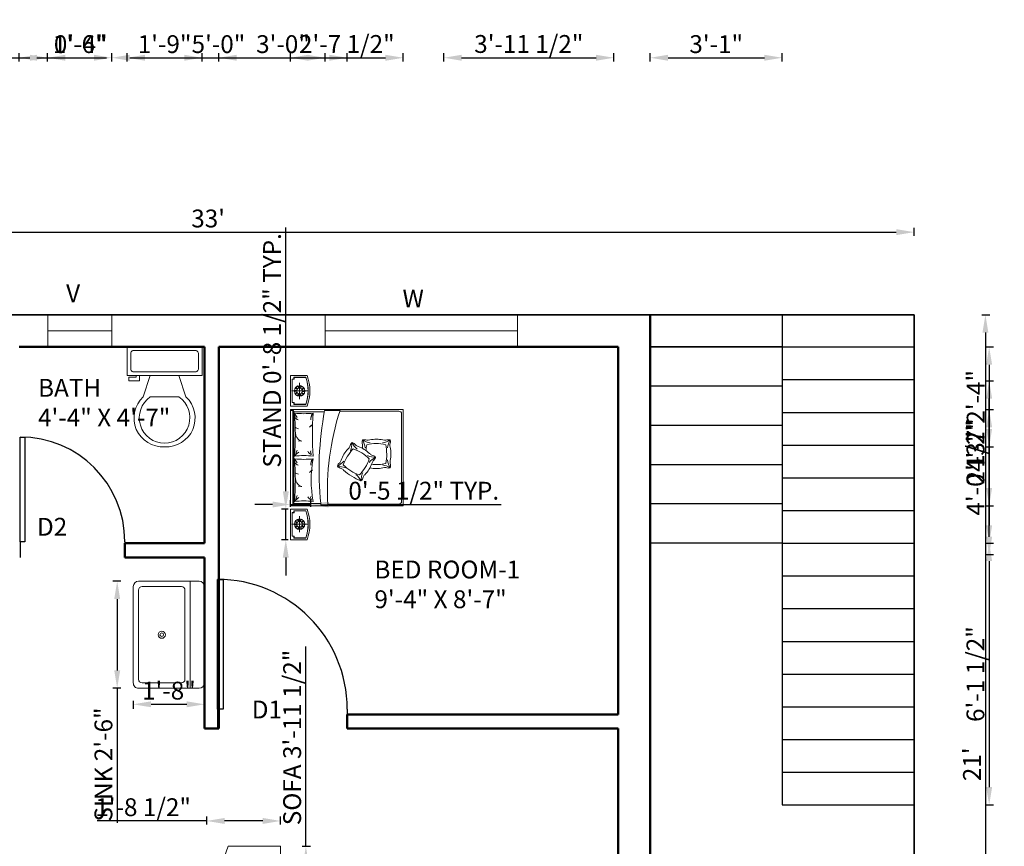
# Model space of a CAD drawing. Units: inches. Extents: x -26 to 423, y -281 to 96.
# Tile 3 of 3: x 147 to 423, y -136 to 96. Entities that reach past the tile are written whole.
import ezdxf

# ---------------------------------------------------------------- set-up
doc = ezdxf.new("R2010")
doc.units = ezdxf.units.IN
doc.header["$PDMODE"] = 35
doc.header["$PDSIZE"] = 5
for name, color, linetype, lineweight in [('A-ANNO-DIMS', 2, 'Continuous', 18), ('A-AREA-IDEN', 7, 'Continuous', 25), ('A-DOOR', 3, 'Continuous', 25), ('A-FLOR-FIXT', 9, 'Continuous', 18), ('A-FLOR-STRS', 7, 'Continuous', 25), ('A-GLAZ', 4, 'Continuous', 18), ('A-WALL', 7, 'Continuous', 50), ('C-PROP', 7, 'Continuous', 35), ('furn', 28, 'Continuous', 18), ('txt', 167, 'Continuous', 18)]:
    doc.layers.add(name, color=color, linetype=linetype, lineweight=lineweight)
doc.styles.get("Standard").update_dxf_attribs({"font": 'arial.ttf'})
doc.dimstyles.new('ISO-25', dxfattribs={"dimtxt": 5, "dimasz": 5, "dimexe": 1.25, "dimexo": 0.625, "dimtad": 1, "dimlunit": 3, "dimtxsty": 'Standard', "dimcen": 2.5, "dimadec": 0, "dimazin": 0, "dimtfac": 1, "dimtmove": 0, "dimatfit": 3, "dimfxl": 1, "dimfxlon": 1, "dimarcsym": 0})

# ---------------------------------------------------------------- blocks, each defined once
blk = doc.blocks.new('*U4')
for p, q in [((9.5, -6), (9.5, -2)), ((-8, -8.5), (-8, -8)), ((-7, -8), (-7, -9.5)), ((-4, -8), (-6, -14)), ((4, -8), (6, -14)), ((-10, -8.5), (-8, -8.5)), ((-10, -9.5), (-10, -8.5)), ((-7, -9.5), (-10, -9.5)), ((4, -14), (-4, -14))]:
    blk.add_line(p, q)
blk.add_lwpolyline([(10.5, -8), (10.5, 0), (-10.5, 0), (-10.5, -8)], close=True)
for points in [[(-9.5, -2), (-9.5, -6)], [(8.5, -1), (-8.5, -1)], [(-8.5, -7), (8.5, -7)]]:
    blk.add_lwpolyline(points)
for centre, radius, start, end in [((-8.625, -1.875), 0.8839, 81.8699, 188.1301), ((8.625, -1.875), 0.8839, 351.8699, 98.1301), ((-8.625, -6.125), 0.8839, 171.869898, 278.1301), ((8.625, -6.125), 0.8839, 261.8699, 8.1301), ((-0.4772, -19.9188), 8.0953, 133.01722, 273.38), ((0.0374, -19.8731), 7.127, 124.50543, 269.7), ((-0.0373, -19.8731), 7.127, 270.3, 55.4946), ((0.4773, -19.9188), 8.0953, 266.62, 46.9828)]:
    blk.add_arc(centre, radius, start, end)
blk = doc.blocks.new('*U2')
for p, q in [((0, 0), (0, -6)), ((40, 0), (40, -6))]:
    blk.add_line(p, q)
blk.add_lwpolyline([(0, 0), (0, 40), (1.75, 40), (1.75, 0)], close=True)
blk.add_arc((0, 0), 40, 0, 90)
blk = doc.blocks.new('Sofa - Roundback 7 ft.')
for p, q in [((-12.00002, -32.4421), (-12.00003, -6.5971)), ((11.99997, -32.4421), (11.99998, -6.5971)), ((-36.000027, -34), (-36.000027, -11.4696)), ((-35.999844, -13.3819), (35.9998, -13.3819)), ((35.99998, -34), (35.99998, -11.4696)), ((-36.000027, -32.4421), (35.99998, -32.4421))]:
    blk.add_line(p, q)
for points in [[(-36.000027, -34), (-42.000027, -34), (-42.000027, -8)], [(41.99998, -8), (41.99998, -34), (35.99998, -34)]]:
    blk.add_lwpolyline(points)
for centre, radius, start, end in [((0, -114.25), 114.25, 68.43141, 111.5686), ((-0.00001, -127.1968), 121.1968, 72.72033, 107.2797)]:
    blk.add_arc(centre, radius, start, end)
blk = doc.blocks.new('Sink-single - 30 in top')
blk.add_line((-15, -3.999996), (15, -3.999996))
for points in [[(-13.5, 0), (13.5, 0)], [(-15, -18.499996), (-15, -1.5)], [(15, -1.5), (15, -18.499996)], [(-12.5, -5.499996), (12.5, -5.499996)], [(-13.5, -17.499996), (-13.5, -6.499996)], [(13.5, -6.499996), (13.5, -17.499996)], [(12.5, -18.499996), (-12.5, -18.499996)], [(13.5, -19.999996), (-13.5, -19.999996)]]:
    blk.add_lwpolyline(points)
for radius in [1, 0.5]:
    blk.add_circle((0, -11.999996), radius)
for centre, radius, start, end in [((-13.5, -1.5), 1.5, 90, 180), ((13.5, -1.5), 1.5, 0, 90), ((-12.5, -6.499996), 1, 90, 180), ((12.5, -6.499996), 1, 0, 90), ((-13.5, -18.499996), 1.5, 180, 270), ((-12.5, -17.499996), 1, 180, 270), ((12.5, -17.499996), 1, 270, 0), ((13.5, -18.499996), 1.5, 270, 0)]:
    blk.add_arc(centre, radius, start, end)
blk = doc.blocks.new('*D12')
at = {"layer": 'A-ANNO-DIMS', "color": 0, "lineweight": -2, "transparency": 16777216}
for p, q in [((1.67, 35.33), (1.67, 37.58)), ((6.67, 36.33), (392.67, 36.33)), ((397.67, 35.33), (397.67, 37.58))]:
    blk.add_line(p, q, dxfattribs=at)
at = {"layer": 'A-ANNO-DIMS', "color": 0, "transparency": 16777216}
for points in [[(6.67, 37.17), (6.67, 35.5), (1.67, 36.33)], [(392.67, 37.17), (392.67, 35.5), (397.67, 36.33)]]:
    blk.add_solid(points, dxfattribs=at)
at = {"layer": 'Defpoints', "color": 0, "transparency": 16777216}
for p in [(397.67, 36.33), (1.67, 13.16), (397.67, 13.16)]:
    blk.add_point(p, dxfattribs=at)
at = {"layer": 'A-ANNO-DIMS', "color": 0, "transparency": 16777216, "insert": (199.67, 39.51), "char_height": 5, "attachment_point": 5}
blk.add_mtext("33'", dxfattribs=at)
blk = doc.blocks.new('*D13')
at = {"layer": 'A-ANNO-DIMS', "color": 0, "lineweight": -2, "transparency": 16777216}
for p, q in [((416.68, 13.16), (418.93, 13.16)), ((417.68, 8.16), (417.68, -233.84)), ((416.68, -238.84), (418.93, -238.84))]:
    blk.add_line(p, q, dxfattribs=at)
at = {"layer": 'A-ANNO-DIMS', "color": 0, "transparency": 16777216}
for points in [[(416.85, 8.16), (418.51, 8.16), (417.68, 13.16)], [(416.85, -233.84), (418.51, -233.84), (417.68, -238.84)]]:
    blk.add_solid(points, dxfattribs=at)
at = {"layer": 'Defpoints', "color": 0, "transparency": 16777216}
for p in [(397.67, 13.16), (397.67, -238.84), (417.68, -238.84)]:
    blk.add_point(p, dxfattribs=at)
at = {"layer": 'A-ANNO-DIMS', "color": 0, "transparency": 16777216, "insert": (414.55, -112.84), "char_height": 5, "attachment_point": 5, "rotation": 90}
blk.add_mtext("21'", dxfattribs=at)
blk = doc.blocks.new('WINDOW-54IN')
blk.add_line((4.5, 54), (4.5, 0))
blk.add_lwpolyline([(0, 54), (9, 54), (9, 0), (0, 0)], close=True)
blk = doc.blocks.new('NIGHTSTAND-COMPACT')
blk.add_lwpolyline([(4.68, 0), (0, 0), (0, 8.58), (4.68, 8.58, -0.181818)], format="xyb", close=True)
for points in [[(0.47, 7.55), (1.03, 7.55), (1.03, 8.11)], [(0.47, 7.6), (0.98, 7.6), (0.98, 8.11)], [(0.47, 0.98), (0.47, 7.6)], [(0.51, 0.98), (0.51, 7.6)], [(0.47, 1.03), (1.03, 1.03), (1.03, 0.47)], [(0.47, 0.98), (0.98, 0.98), (0.98, 0.47)]]:
    blk.add_lwpolyline(points)
for points in [[(0.98, 8.11), (4.35, 8.11, -0.167087), (4.35, 0.47), (0.98, 0.47)], [(0.98, 8.06), (4.32, 8.06, -0.165559), (4.32, 0.51), (0.98, 0.51)]]:
    blk.add_lwpolyline(points, format="xyb")
blk = doc.blocks.new('*D21')
at = {"layer": 'A-ANNO-DIMS', "color": 0, "lineweight": -2, "transparency": 16777216}
for p, q in [((221.46, -36.3), (221.46, 37.67)), ((222.12, -41.3), (220.21, -41.3)), ((221.46, -49.88), (221.46, -41.3)), ((222.12, -49.88), (220.21, -49.88)), ((221.46, -54.88), (221.46, -59.88))]:
    blk.add_line(p, q, dxfattribs=at)
at = {"layer": 'A-ANNO-DIMS', "color": 0, "transparency": 16777216}
for points in [[(220.62, -36.3), (222.29, -36.3), (221.46, -41.3)], [(220.62, -54.88), (222.29, -54.88), (221.46, -49.88)]]:
    blk.add_solid(points, dxfattribs=at)
at = {"layer": 'Defpoints', "color": 0, "transparency": 16777216}
for p in [(221.46, -41.3), (222.74, -41.3), (222.74, -49.88)]:
    blk.add_point(p, dxfattribs=at)
at = {"layer": 'A-ANNO-DIMS', "color": 0, "transparency": 16777216, "insert": (218.25, 3.18), "char_height": 5, "attachment_point": 5, "rotation": 90}
blk.add_mtext('STAND 0\'-8 1/2" TYP.', dxfattribs=at)
blk = doc.blocks.new('*D22')
at = {"layer": 'A-ANNO-DIMS', "color": 0, "lineweight": -2, "transparency": 16777216}
for p, q in [((217.74, -40.01), (212.74, -40.01)), ((222.74, -40.67), (222.74, -38.76)), ((222.74, -40.01), (228.46, -40.01)), ((228.46, -40.67), (228.46, -38.76)), ((233.46, -40.01), (281.84, -40.01))]:
    blk.add_line(p, q, dxfattribs=at)
at = {"layer": 'A-ANNO-DIMS', "color": 0, "transparency": 16777216}
for points in [[(217.74, -39.18), (217.74, -40.85), (222.74, -40.01)], [(233.46, -39.18), (233.46, -40.85), (228.46, -40.01)]]:
    blk.add_solid(points, dxfattribs=at)
at = {"layer": 'Defpoints', "color": 0, "transparency": 16777216}
for p in [(222.74, -41.3), (228.46, -40.01), (228.46, -41.3)]:
    blk.add_point(p, dxfattribs=at)
at = {"layer": 'A-ANNO-DIMS', "color": 0, "transparency": 16777216, "insert": (260.15, -36.8), "char_height": 5, "attachment_point": 5}
blk.add_mtext('0\'-5 1/2" TYP.', dxfattribs=at)
blk = doc.blocks.new('*D23')
at = {"layer": 'A-ANNO-DIMS', "color": 0, "lineweight": -2, "transparency": 16777216}
for p, q in [((227.09, -135.82), (227.09, -79.81)), ((226.09, -135.82), (228.34, -135.82)), ((227.09, -178.2), (227.09, -140.82)), ((226.09, -183.2), (228.34, -183.2))]:
    blk.add_line(p, q, dxfattribs=at)
at = {"layer": 'A-ANNO-DIMS', "color": 0, "transparency": 16777216}
for points in [[(226.26, -140.82), (227.92, -140.82), (227.09, -135.82)], [(226.26, -178.2), (227.92, -178.2), (227.09, -183.2)]]:
    blk.add_solid(points, dxfattribs=at)
at = {"layer": 'Defpoints', "color": 0, "transparency": 16777216}
for p in [(219.98, -135.82), (227.09, -135.82), (219.98, -183.2)]:
    blk.add_point(p, dxfattribs=at)
at = {"layer": 'A-ANNO-DIMS', "color": 0, "transparency": 16777216, "insert": (223.88, -105.32), "char_height": 5, "attachment_point": 5, "rotation": 90}
blk.add_mtext('SOFA 3\'-11 1/2"', dxfattribs=at)
blk = doc.blocks.new('*D24')
at = {"layer": 'A-ANNO-DIMS', "color": 0, "lineweight": -2, "transparency": 16777216}
for p, q in [((199.3, -128.72), (168.58, -128.72)), ((199.3, -129.72), (199.3, -127.47)), ((214.98, -128.72), (204.3, -128.72)), ((219.98, -129.72), (219.98, -127.47))]:
    blk.add_line(p, q, dxfattribs=at)
at = {"layer": 'A-ANNO-DIMS', "color": 0, "transparency": 16777216}
for points in [[(204.3, -127.88), (204.3, -129.55), (199.3, -128.72)], [(214.98, -127.88), (214.98, -129.55), (219.98, -128.72)]]:
    blk.add_solid(points, dxfattribs=at)
at = {"layer": 'Defpoints', "color": 0, "transparency": 16777216}
for p in [(199.3, -128.72), (199.3, -135.82), (219.98, -135.82)]:
    blk.add_point(p, dxfattribs=at)
at = {"layer": 'A-ANNO-DIMS', "color": 0, "transparency": 16777216, "insert": (181.44, -125.51), "char_height": 5, "attachment_point": 5}
blk.add_mtext('1\'-8 1/2"', dxfattribs=at)
blk = doc.blocks.new('*D27')
at = {"layer": 'A-ANNO-DIMS', "color": 0, "lineweight": -2, "transparency": 16777216}
for p, q in [((175.17, -61.52), (172.92, -61.52)), ((174.17, -66.52), (174.17, -86.52)), ((175.17, -91.52), (172.92, -91.52)), ((174.17, -91.52), (174.17, -129.28))]:
    blk.add_line(p, q, dxfattribs=at)
at = {"layer": 'A-ANNO-DIMS', "color": 0, "transparency": 16777216}
for points in [[(173.34, -66.52), (175.01, -66.52), (174.17, -61.52)], [(173.34, -86.52), (175.01, -86.52), (174.17, -91.52)]]:
    blk.add_solid(points, dxfattribs=at)
at = {"layer": 'Defpoints', "color": 0, "transparency": 16777216}
for p in [(178.67, -61.52), (174.17, -91.52), (178.67, -91.52)]:
    blk.add_point(p, dxfattribs=at)
at = {"layer": 'A-ANNO-DIMS', "color": 0, "transparency": 16777216, "insert": (170.96, -112.9), "char_height": 5, "attachment_point": 5, "rotation": 90}
blk.add_mtext('SINK 2\'-6"', dxfattribs=at)
blk = doc.blocks.new('*D28')
at = {"layer": 'A-ANNO-DIMS', "color": 0, "lineweight": -2, "transparency": 16777216}
for p, q in [((178.67, -95.02), (178.67, -97.27)), ((183.67, -96.02), (193.67, -96.02)), ((198.67, -95.02), (198.67, -97.27))]:
    blk.add_line(p, q, dxfattribs=at)
at = {"layer": 'A-ANNO-DIMS', "color": 0, "transparency": 16777216}
for points in [[(183.67, -95.19), (183.67, -96.85), (178.67, -96.02)], [(193.67, -95.19), (193.67, -96.85), (198.67, -96.02)]]:
    blk.add_solid(points, dxfattribs=at)
at = {"layer": 'Defpoints', "color": 0, "transparency": 16777216}
for p in [(178.67, -91.52), (198.67, -91.52), (198.67, -96.02)]:
    blk.add_point(p, dxfattribs=at)
at = {"layer": 'A-ANNO-DIMS', "color": 0, "transparency": 16777216, "insert": (188.67, -92.84), "char_height": 5, "attachment_point": 5}
blk.add_mtext('1\'-8"', dxfattribs=at)
blk = doc.blocks.new('*D33')
at = {"layer": 'A-ANNO-DIMS', "color": 0, "lineweight": -2, "transparency": 16777216}
for p, q in [((1.67, 84.21), (1.67, 86.46)), ((154.67, 84.21), (154.67, 86.46)), ((6.67, 85.21), (149.67, 85.21))]:
    blk.add_line(p, q, dxfattribs=at)
at = {"layer": 'A-ANNO-DIMS', "color": 0, "transparency": 16777216}
for points in [[(6.67, 86.05), (6.67, 84.38), (1.67, 85.21)], [(149.67, 86.05), (149.67, 84.38), (154.67, 85.21)]]:
    blk.add_solid(points, dxfattribs=at)
at = {"layer": 'Defpoints', "color": 0, "transparency": 16777216}
for p in [(154.67, 85.21), (1.67, 13.16), (154.67, 13.16)]:
    blk.add_point(p, dxfattribs=at)
at = {"layer": 'A-ANNO-DIMS', "color": 0, "transparency": 16777216, "insert": (78.17, 88.39), "char_height": 5, "attachment_point": 5}
blk.add_mtext('12\'-9"', dxfattribs=at)
blk = doc.blocks.new('*D34')
at = {"layer": 'A-ANNO-DIMS', "color": 0, "lineweight": -2, "transparency": 16777216}
for p, q in [((154.67, 84.21), (154.67, 86.46)), ((172.67, 84.21), (172.67, 86.46)), ((159.67, 85.21), (167.67, 85.21))]:
    blk.add_line(p, q, dxfattribs=at)
at = {"layer": 'A-ANNO-DIMS', "color": 0, "transparency": 16777216}
for points in [[(159.67, 86.05), (159.67, 84.38), (154.67, 85.21)], [(167.67, 86.05), (167.67, 84.38), (172.67, 85.21)]]:
    blk.add_solid(points, dxfattribs=at)
at = {"layer": 'Defpoints', "color": 0, "transparency": 16777216}
for p in [(172.67, 85.21), (154.67, 13.16), (172.67, 13.16)]:
    blk.add_point(p, dxfattribs=at)
at = {"layer": 'A-ANNO-DIMS', "color": 0, "transparency": 16777216, "insert": (163.67, 88.39), "char_height": 5, "attachment_point": 5}
blk.add_mtext('1\'-6"', dxfattribs=at)
blk = doc.blocks.new('*D35')
at = {"layer": 'A-ANNO-DIMS', "color": 0, "lineweight": -2, "transparency": 16777216}
for p, q in [((172.67, 84.21), (172.67, 86.46)), ((232.46, 84.21), (232.46, 86.46)), ((177.67, 85.21), (227.46, 85.21))]:
    blk.add_line(p, q, dxfattribs=at)
at = {"layer": 'A-ANNO-DIMS', "color": 0, "transparency": 16777216}
for points in [[(177.67, 86.05), (177.67, 84.38), (172.67, 85.21)], [(227.46, 86.05), (227.46, 84.38), (232.46, 85.21)]]:
    blk.add_solid(points, dxfattribs=at)
at = {"layer": 'Defpoints', "color": 0, "transparency": 16777216}
for p in [(232.46, 85.21), (172.67, 13.16), (232.46, 13.16)]:
    blk.add_point(p, dxfattribs=at)
at = {"layer": 'A-ANNO-DIMS', "color": 0, "transparency": 16777216, "insert": (202.56, 88.39), "char_height": 5, "attachment_point": 5}
blk.add_mtext('5\'-0"', dxfattribs=at)
blk = doc.blocks.new('*D37')
at = {"layer": 'A-ANNO-DIMS', "color": 0, "lineweight": -2, "transparency": 16777216}
for p, q in [((202.67, 84.21), (202.67, 86.46)), ((238.67, 84.21), (238.67, 86.46)), ((207.67, 85.21), (233.67, 85.21))]:
    blk.add_line(p, q, dxfattribs=at)
at = {"layer": 'A-ANNO-DIMS', "color": 0, "transparency": 16777216}
for points in [[(207.67, 86.05), (207.67, 84.38), (202.67, 85.21)], [(233.67, 86.05), (233.67, 84.38), (238.67, 85.21)]]:
    blk.add_solid(points, dxfattribs=at)
at = {"layer": 'Defpoints', "color": 0, "transparency": 16777216}
for p in [(238.67, 85.21), (202.67, -102.84), (238.67, -102.84)]:
    blk.add_point(p, dxfattribs=at)
at = {"layer": 'A-ANNO-DIMS', "color": 0, "transparency": 16777216, "insert": (220.67, 88.39), "char_height": 5, "attachment_point": 5}
blk.add_mtext('3\'-0"', dxfattribs=at)
blk = doc.blocks.new('*D38')
at = {"layer": 'A-ANNO-DIMS', "color": 0, "lineweight": -2, "transparency": 16777216}
for p, q in [((146.98, -259.17), (146.98, -261.42)), ((176.32, -259.17), (176.32, -261.42)), ((151.98, -260.17), (171.32, -260.17))]:
    blk.add_line(p, q, dxfattribs=at)
at = {"layer": 'A-ANNO-DIMS', "color": 0, "transparency": 16777216}
for points in [[(151.98, -259.33), (151.98, -261), (146.98, -260.17)], [(171.32, -259.33), (171.32, -261), (176.32, -260.17)]]:
    blk.add_solid(points, dxfattribs=at)
at = {"layer": 'Defpoints', "color": 0, "transparency": 16777216}
for p in [(146.98, -50.44), (176.32, -50.84), (176.32, -260.17)]:
    blk.add_point(p, dxfattribs=at)
at = {"layer": 'A-ANNO-DIMS', "color": 0, "transparency": 16777216, "insert": (161.65, -256.96), "char_height": 5, "attachment_point": 5}
blk.add_mtext('2\'-5 1/2"', dxfattribs=at)
blk = doc.blocks.new('*D39')
at = {"layer": 'A-ANNO-DIMS', "color": 0, "lineweight": -2, "transparency": 16777216}
for p, q in [((265.77, 84.21), (265.77, 86.46)), ((313.46, 84.21), (313.46, 86.46)), ((270.77, 85.21), (308.46, 85.21))]:
    blk.add_line(p, q, dxfattribs=at)
at = {"layer": 'A-ANNO-DIMS', "color": 0, "transparency": 16777216}
for points in [[(270.77, 86.05), (270.77, 84.38), (265.77, 85.21)], [(308.46, 86.05), (308.46, 84.38), (313.46, 85.21)]]:
    blk.add_solid(points, dxfattribs=at)
at = {"layer": 'Defpoints', "color": 0, "transparency": 16777216}
for p in [(313.46, 85.21), (265.77, -229.84), (313.46, -229.84)]:
    blk.add_point(p, dxfattribs=at)
at = {"layer": 'A-ANNO-DIMS', "color": 0, "transparency": 16777216, "insert": (289.61, 88.43), "char_height": 5, "attachment_point": 5}
blk.add_mtext('3\'-11 1/2"', dxfattribs=at)
blk = doc.blocks.new('*D41')
at = {"layer": 'A-ANNO-DIMS', "color": 0, "lineweight": -2, "transparency": 16777216}
for p, q in [((323.67, 84.21), (323.67, 86.46)), ((360.67, 84.21), (360.67, 86.46)), ((328.67, 85.21), (355.67, 85.21))]:
    blk.add_line(p, q, dxfattribs=at)
at = {"layer": 'A-ANNO-DIMS', "color": 0, "transparency": 16777216}
for points in [[(328.67, 86.05), (328.67, 84.38), (323.67, 85.21)], [(355.67, 86.05), (355.67, 84.38), (360.67, 85.21)]]:
    blk.add_solid(points, dxfattribs=at)
at = {"layer": 'Defpoints', "color": 0, "transparency": 16777216}
for p in [(360.67, 85.21), (323.67, 13.16), (360.67, 13.16)]:
    blk.add_point(p, dxfattribs=at)
at = {"layer": 'A-ANNO-DIMS', "color": 0, "transparency": 16777216, "insert": (342.17, 88.39), "char_height": 5, "attachment_point": 5}
blk.add_mtext('3\'-1"', dxfattribs=at)
blk = doc.blocks.new('*D42')
at = {"layer": 'A-ANNO-DIMS', "color": 0, "lineweight": -2, "transparency": 16777216}
for p, q in [((417.73, 4.16), (419.98, 4.16)), ((418.73, -0.84), (418.73, -45.86)), ((417.73, -50.86), (419.98, -50.86))]:
    blk.add_line(p, q, dxfattribs=at)
at = {"layer": 'A-ANNO-DIMS', "color": 0, "transparency": 16777216}
for points in [[(417.89, -0.84), (419.56, -0.84), (418.73, 4.16)], [(417.89, -45.86), (419.56, -45.86), (418.73, -50.86)]]:
    blk.add_solid(points, dxfattribs=at)
at = {"layer": 'Defpoints', "color": 0, "transparency": 16777216}
for p in [(397.67, 4.16), (397.67, -50.86), (418.73, -50.86)]:
    blk.add_point(p, dxfattribs=at)
at = {"layer": 'A-ANNO-DIMS', "color": 0, "transparency": 16777216, "insert": (415.6, -23.35), "char_height": 5, "attachment_point": 5, "rotation": 90}
blk.add_mtext('4\'-7"', dxfattribs=at)
blk = doc.blocks.new('*D43')
at = {"layer": 'A-ANNO-DIMS', "color": 0, "lineweight": -2, "transparency": 16777216}
for p, q in [((417.73, -50.86), (419.98, -50.86)), ((418.73, -55.86), (418.73, -119.23)), ((417.73, -124.23), (419.98, -124.23))]:
    blk.add_line(p, q, dxfattribs=at)
at = {"layer": 'A-ANNO-DIMS', "color": 0, "transparency": 16777216}
for points in [[(417.89, -55.86), (419.56, -55.86), (418.73, -50.86)], [(417.89, -119.23), (419.56, -119.23), (418.73, -124.23)]]:
    blk.add_solid(points, dxfattribs=at)
at = {"layer": 'Defpoints', "color": 0, "transparency": 16777216}
for p in [(397.67, -50.86), (397.67, -124.23), (418.73, -124.23)]:
    blk.add_point(p, dxfattribs=at)
at = {"layer": 'A-ANNO-DIMS', "color": 0, "transparency": 16777216, "insert": (415.52, -87.55), "char_height": 5, "attachment_point": 5, "rotation": 90}
blk.add_mtext('6\'-1 1/2"', dxfattribs=at)
blk = doc.blocks.new('*D47')
at = {"layer": 'A-ANNO-DIMS', "color": 0, "lineweight": -2, "transparency": 16777216}
for p, q in [((417.73, -5.34), (419.98, -5.34)), ((418.73, -49.07), (418.73, -10.34)), ((417.73, -54.07), (419.98, -54.07))]:
    blk.add_line(p, q, dxfattribs=at)
at = {"layer": 'A-ANNO-DIMS', "color": 0, "transparency": 16777216}
for points in [[(417.89, -10.34), (419.56, -10.34), (418.73, -5.34)], [(417.89, -49.07), (419.56, -49.07), (418.73, -54.07)]]:
    blk.add_solid(points, dxfattribs=at)
at = {"layer": 'Defpoints', "color": 0, "transparency": 16777216}
for p in [(82.79, -5.34), (418.73, -5.34), (82.79, -54.07)]:
    blk.add_point(p, dxfattribs=at)
at = {"layer": 'A-ANNO-DIMS', "color": 0, "transparency": 16777216, "insert": (415.52, -29.71), "char_height": 5, "attachment_point": 5, "rotation": 90}
blk.add_mtext('4\'-0 1/2"', dxfattribs=at)
blk = doc.blocks.new('*D48')
at = {"layer": 'A-ANNO-DIMS', "color": 0, "lineweight": -2, "transparency": 16777216}
for p, q in [((222.74, 84.21), (222.74, 86.46)), ((254.41, 84.21), (254.41, 86.46)), ((227.74, 85.21), (249.41, 85.21))]:
    blk.add_line(p, q, dxfattribs=at)
at = {"layer": 'A-ANNO-DIMS', "color": 0, "transparency": 16777216}
for points in [[(227.74, 86.05), (227.74, 84.38), (222.74, 85.21)], [(249.41, 86.05), (249.41, 84.38), (254.41, 85.21)]]:
    blk.add_solid(points, dxfattribs=at)
at = {"layer": 'Defpoints', "color": 0, "transparency": 16777216}
for p in [(254.41, 85.21), (222.74, -13.38), (254.41, -13.38)]:
    blk.add_point(p, dxfattribs=at)
at = {"layer": 'A-ANNO-DIMS', "color": 0, "transparency": 16777216, "insert": (238.57, 88.42), "char_height": 5, "attachment_point": 5}
blk.add_mtext('2\'-7 1/2"', dxfattribs=at)
blk = doc.blocks.new('*D49')
at = {"layer": 'A-ANNO-DIMS', "color": 0, "lineweight": -2, "transparency": 16777216}
for p, q in [((417.73, -13.38), (419.98, -13.38)), ((418.73, -35.36), (418.73, -18.38)), ((417.73, -40.36), (419.98, -40.36))]:
    blk.add_line(p, q, dxfattribs=at)
at = {"layer": 'A-ANNO-DIMS', "color": 0, "transparency": 16777216}
for points in [[(417.89, -18.38), (419.56, -18.38), (418.73, -13.38)], [(417.89, -35.36), (419.56, -35.36), (418.73, -40.36)]]:
    blk.add_solid(points, dxfattribs=at)
at = {"layer": 'Defpoints', "color": 0, "transparency": 16777216}
for p in [(254.41, -13.38), (418.73, -13.38), (254.41, -40.36)]:
    blk.add_point(p, dxfattribs=at)
at = {"layer": 'A-ANNO-DIMS', "color": 0, "transparency": 16777216, "insert": (415.55, -26.87), "char_height": 5, "attachment_point": 5, "rotation": 90}
blk.add_mtext('2\'-3"', dxfattribs=at)
blk = doc.blocks.new('*D51')
at = {"layer": 'A-ANNO-DIMS', "color": 0, "lineweight": -2, "transparency": 16777216}
for p, q in [((-18.38, -3.86), (-20.63, -3.86)), ((-19.38, -44.88), (-19.38, -8.86)), ((-18.38, -49.88), (-20.63, -49.88))]:
    blk.add_line(p, q, dxfattribs=at)
at = {"layer": 'A-ANNO-DIMS', "color": 0, "transparency": 16777216}
for points in [[(-20.22, -8.86), (-18.55, -8.86), (-19.38, -3.86)], [(-20.22, -44.88), (-18.55, -44.88), (-19.38, -49.88)]]:
    blk.add_solid(points, dxfattribs=at)
at = {"layer": 'Defpoints', "color": 0, "transparency": 16777216}
for p in [(-19.38, -3.86), (222.74, -3.86), (222.74, -49.88)]:
    blk.add_point(p, dxfattribs=at)
at = {"layer": 'A-ANNO-DIMS', "color": 0, "transparency": 16777216, "insert": (-22.56, -26.87), "char_height": 5, "attachment_point": 5, "rotation": 90}
blk.add_mtext('3\'-10"', dxfattribs=at)
blk = doc.blocks.new('*D52')
at = {"layer": 'A-ANNO-DIMS', "color": 0, "lineweight": -2, "transparency": 16777216}
for p, q in [((176.96, 84.21), (176.96, 86.46)), ((197.96, 84.21), (197.96, 86.46)), ((181.96, 85.21), (192.96, 85.21))]:
    blk.add_line(p, q, dxfattribs=at)
at = {"layer": 'A-ANNO-DIMS', "color": 0, "transparency": 16777216}
for points in [[(181.96, 86.05), (181.96, 84.38), (176.96, 85.21)], [(192.96, 86.05), (192.96, 84.38), (197.96, 85.21)]]:
    blk.add_solid(points, dxfattribs=at)
at = {"layer": 'Defpoints', "color": 0, "transparency": 16777216}
for p in [(197.96, 85.21), (176.96, 4.16), (197.96, 4.16)]:
    blk.add_point(p, dxfattribs=at)
at = {"layer": 'A-ANNO-DIMS', "color": 0, "transparency": 16777216, "insert": (187.46, 88.39), "char_height": 5, "attachment_point": 5}
blk.add_mtext('1\'-9"', dxfattribs=at)
blk = doc.blocks.new('*D53')
at = {"layer": 'A-ANNO-DIMS', "color": 0, "lineweight": -2, "transparency": 16777216}
for p, q in [((417.73, 4.16), (419.98, 4.16)), ((418.73, -0.84), (418.73, -18.84)), ((417.73, -23.84), (419.98, -23.84))]:
    blk.add_line(p, q, dxfattribs=at)
at = {"layer": 'A-ANNO-DIMS', "color": 0, "transparency": 16777216}
for points in [[(417.89, -0.84), (419.56, -0.84), (418.73, 4.16)], [(417.89, -18.84), (419.56, -18.84), (418.73, -23.84)]]:
    blk.add_solid(points, dxfattribs=at)
at = {"layer": 'Defpoints', "color": 0, "transparency": 16777216}
for p in [(197.96, 4.16), (187.46, -23.84), (418.73, -23.84)]:
    blk.add_point(p, dxfattribs=at)
at = {"layer": 'A-ANNO-DIMS', "color": 0, "transparency": 16777216, "insert": (415.59, -9.84), "char_height": 5, "attachment_point": 5, "rotation": 90}
blk.add_mtext('2\'-4"', dxfattribs=at)
blk = doc.blocks.new('*D54')
at = {"layer": 'A-ANNO-DIMS', "color": 0, "lineweight": -2, "transparency": 16777216}
for p, q in [((142.67, 84.21), (142.67, 86.46)), ((146.67, 84.21), (146.67, 86.46)), ((137.67, 85.21), (132.67, 85.21)), ((142.67, 85.21), (146.67, 85.21)), ((151.67, 85.21), (171.21, 85.21))]:
    blk.add_line(p, q, dxfattribs=at)
at = {"layer": 'A-ANNO-DIMS', "color": 0, "transparency": 16777216}
for points in [[(137.67, 86.05), (137.67, 84.38), (142.67, 85.21)], [(151.67, 86.05), (151.67, 84.38), (146.67, 85.21)]]:
    blk.add_solid(points, dxfattribs=at)
at = {"layer": 'Defpoints', "color": 0, "transparency": 16777216}
for p in [(146.67, 85.21), (142.67, 4.16), (146.67, 4.16)]:
    blk.add_point(p, dxfattribs=at)
at = {"layer": 'A-ANNO-DIMS', "color": 0, "transparency": 16777216, "insert": (163.94, 88.39), "char_height": 5, "attachment_point": 5}
blk.add_mtext('0\'-4"', dxfattribs=at)

msp = doc.modelspace()

# ---------------------------------------------------------------- linework, layer by layer
at = {"layer": 'A-FLOR-STRS'}
for p, q in [((360.673, 13.158), (360.673, -124.228)), ((323.673, 4.158), (397.673, 4.158)), ((360.673, 4.158), (323.673, 4.158)), ((360.673, 4.158), (397.673, 4.158)), ((360.673, -5.012), (397.673, -5.012)), ((360.673, -6.846), (323.673, -6.846)), ((360.673, -14.183), (397.673, -14.183)), ((360.673, -17.851), (323.673, -17.851)), ((360.673, -23.353), (397.673, -23.353)), ((360.673, -28.856), (323.673, -28.856)), ((360.673, -32.524), (397.673, -32.524)), ((360.673, -39.86), (323.673, -39.86)), ((360.673, -41.694), (397.673, -41.694)), ((360.673, -50.865), (323.673, -50.865)), ((360.673, -50.865), (397.673, -50.865)), ((360.673, -60.035), (397.673, -60.035)), ((360.673, -69.205), (397.673, -69.205)), ((360.673, -78.376), (397.673, -78.376)), ((360.673, -87.546), (397.673, -87.546)), ((360.673, -96.717), (397.673, -96.717)), ((360.673, -105.887), (397.673, -105.887)), ((360.673, -115.058), (397.673, -115.058)), ((360.673, -124.228), (397.673, -124.228))]:
    msp.add_line(p, q, dxfattribs=at)
at = {"layer": 'A-GLAZ'}
for p, q in [((154.673, 4.158), (154.673, 13.158)), ((172.673, 4.158), (172.673, 13.158)), ((154.673, 8.658), (172.673, 8.658))]:
    msp.add_line(p, q, dxfattribs=at)
at = {"layer": 'A-WALL'}
for p, q in [((323.673, -181.842), (323.673, 13.158)), ((146.673, 4.158), (198.673, 4.158)), ((198.673, -50.842), (198.673, 4.158)), ((202.673, -102.842), (202.673, 4.158)), ((202.673, 4.158), (314.673, 4.158)), ((314.673, -98.842), (314.673, 4.158)), ((176.324, -50.842), (198.673, -50.842)), ((176.324, -50.842), (176.324, -54.842)), ((176.324, -54.842), (198.673, -54.842)), ((198.673, -102.842), (198.673, -54.842)), ((238.673, -98.842), (314.673, -98.842)), ((238.673, -102.842), (238.673, -98.842)), ((202.673, -102.842), (198.673, -102.842)), ((238.673, -102.842), (314.673, -102.842)), ((314.673, -181.842), (314.673, -102.842))]:
    msp.add_line(p, q, dxfattribs=at)
at = {"layer": 'C-PROP'}
for p, q in [((1.673, 13.158), (397.673, 13.158)), ((397.673, 13.158), (397.673, -238.842))]:
    msp.add_line(p, q, dxfattribs=at)
at = {"layer": 'furn'}
for p, q in [((227.577, -8.198), (223.078, -8.198)), ((225.327, -5.948), (225.327, -10.447)), ((223.473, -13.996), (232.277, -13.996)), ((223.706, -39.896), (223.706, -13.847)), ((223.473, -39.763), (231.264, -39.763)), ((225.327, -47.794), (225.327, -43.296)), ((227.576, -45.545), (223.078, -45.545))]:
    msp.add_line(p, q, dxfattribs=at)
for points in [[(222.742, -40.364), (254.406, -40.364), (254.406, -13.379), (222.742, -13.379)], [(222.742, -13.63), (223.473, -13.63), (223.473, -40.208), (222.742, -40.208), (222.742, -13.379)]]:
    msp.add_lwpolyline(points, dxfattribs=at)
for points in [[(231.264, -40.128), (231.264, -39.763, -0.0729439), (232.353, -13.63), (236.679, -13.63, 0.0925678), (233.249, -40.128)], [(229.133, -26.447, 0.0585956), (223.92, -26.447, 0.0366479), (223.92, -14.424, 0.052163), (229.133, -14.424, 0.0369674)], [(229.133, -39.168, 0.0585956), (223.92, -39.168, 0.0368889), (223.92, -27.223, 0.052163), (229.133, -27.223, 0.0931113)]]:
    msp.add_lwpolyline(points, format="xyb", close=True, dxfattribs=at)
for points in [[(233.235, -39.896), (253.158, -39.896, 0.4142136), (253.938, -39.116), (253.938, -14.627, 0.4142136), (253.158, -13.847), (236.602, -13.847)], [(250.751, -21.923, 0.1594612), (249.522, -21.977, -0.0762829), (248.703, -21.923, 0.1150751), (245, -21.923, -0.0762829), (244.181, -21.977, 0.1594612), (242.952, -21.923)], [(243.751, -24.115, 0.0912961), (242.952, -21.923, 0.0912961), (245.142, -22.729, 0.0912961)], [(248.561, -22.729, 0.0912961), (250.751, -21.923, 0.0912961), (249.952, -24.115)], [(242.108, -31.7, 0.1110065), (244.878, -27.244, 0.1195491), (240.371, -24.435, 0.1078134), (237.588, -28.877)], [(239.562, -24.957, 0.0912961), (240.043, -22.674, 0.0912961), (241.475, -24.516, 0.0912961)], [(246.662, -26.798, 0.1594612), (245.591, -26.194, -0.0762829), (244.924, -25.715, 0.1150751), (241.782, -23.757, -0.0762829), (241.057, -23.369, 0.1594612), (240.043, -22.674)], [(249.477, -28.491, 0.1110065), (249.473, -23.244, 0.1195491), (244.161, -23.244, 0.0332124), (243.916, -24.858)], [(244.377, -26.324, 0.0912961), (246.662, -26.798, 0.0912961), (244.825, -28.237)], [(249.952, -27.529, 0.0912961), (250.751, -29.722, 0.0912961), (248.561, -28.916, 0.0912961)], [(238.204, -29.767, 0.0912961), (235.918, -29.293, 0.0912961), (237.756, -27.855, 0.0912961)], [(237.594, -28.901, 0.1218652), (242.107, -31.699, 0.1218652)], [(243.019, -31.134, 0.0912961), (242.538, -33.418, 0.0912961), (241.105, -31.575, 0.0912961)]]:
    msp.add_lwpolyline(points, format="xyb", dxfattribs=at)
for centre, radius in [((225.327, -8.198), 1.469), ((225.327, -8.198), 0.796), ((225.327, -45.545), 1.469), ((225.327, -45.545), 0.796)]:
    msp.add_circle(centre, radius, dxfattribs=at)
for centre, radius, start, end in [((224.513, -8.95), 0.944, 87.51025, 133.82997), ((224.476, -8.863), 0.72, 85.46198, 145.69983), ((224.247, -8.236), 0.72, 49.46198, 109.69983), ((224.186, -8.221), 0.944, 51.51025, 97.82997), ((224.391, -7.486), 0.72, 13.46198, 73.69983), ((224.32, -7.549), 0.944, 15.51025, 61.82997), ((224.917, -7.075), 0.72, 337.46198, 37.69983), ((224.823, -7.084), 0.944, 339.51025, 25.82997), ((225.625, -7.159), 0.72, 301.46198, 1.69983), ((225.544, -7.111), 0.944, 303.51025, 349.82997), ((226.141, -7.445), 0.944, 267.51025, 313.82997), ((226.179, -7.532), 0.72, 265.46198, 325.69983), ((225.111, -9.285), 0.944, 123.51025, 169.82997), ((225.03, -9.237), 0.72, 121.46198, 181.69983), ((225.791, -9.204), 0.944, 159.51025, 205.82997), ((225.697, -9.213), 0.72, 157.46198, 217.69983), ((226.294, -8.739), 0.944, 195.51025, 241.82997), ((226.224, -8.802), 0.72, 193.46198, 253.69983), ((226.428, -8.067), 0.944, 231.51025, 277.82997), ((226.407, -8.16), 0.72, 229.46198, 289.69983), ((223.238, -13.847), 0.468, 0, 90), ((227.493, -12.864), 3.931, 204.64565, 224.15848), ((225.655, -14.225), 2.182, 220.53543, 250.35581), ((230.625, -16.026), 2.132, 134.40604, 186.83423), ((229.881, -15.628), 1.351, 123.63488, 180.84559), ((225.367, -16.789), 2.028, 231.81741, 259.89867), ((232.759, -22.932), 6.512, 126.20852, 135.08491), ((228.912, -18.115), 0.437, 83.75428, 167.21866), ((227.011, -19.713), 2.891, 186.68493, 238.3182), ((244.682, -22.505), 1.826, 161.39955, 201.57741), ((248.541, -22.404), 2.262, 340.70232, 12.28404), ((219.562, -23.675), 5.165, 327.53791, 347.5233), ((225.402, -23.466), 1.295, 65.89274, 106.11919), ((244.706, -30.174), 8.15, 135.13065, 161.38844), ((236.99, -22.535), 2.708, 315.77185, 333.2208), ((241.204, -24.083), 1.826, 129.47264, 169.6505), ((250.876, -25.822), 8.15, 167.05756, 168.7033), ((240.287, -23.42), 2.708, 347.69876, 5.14771), ((253.375, -23.377), 2.708, 175.2252, 192.67415), ((242.801, -25.848), 8.15, 347.05756, 13.31535), ((228.795, -30.356), 6.248, 126.49353, 141.27919), ((227.493, -25.584), 3.931, 204.64565, 224.15848), ((229.253, -24.394), 1.733, 204.2916, 250.9896), ((229.615, -25.294), 1.185, 166.48229, 218.55627), ((230.625, -28.746), 2.132, 134.40604, 186.83423), ((229.881, -28.348), 1.351, 123.63488, 180.84559), ((234.426, -26.68), 2.708, 323.29829, 340.74724), ((244.532, -26.038), 2.262, 308.77541, 340.35713), ((225.655, -26.945), 2.182, 220.53543, 250.35581), ((237.753, -29.816), 1.908, 127.29372, 164.09733), ((237.377, -27.958), 1.977, 222.46578, 258.70648), ((235.762, -32.311), 2.708, 45.58539, 63.03435), ((237.839, -25.926), 8.15, 315.13065, 341.38844), ((246.851, -21.785), 8.15, 256.87111, 283.12889), ((246.797, -17.764), 11.057, 263.19556, 284.02838), ((248.12, -29.42), 2.708, 143.29829, 160.74724), ((249.288, -32.366), 2.708, 85.03874, 102.4877), ((250.219, -27.818), 1.977, 249.36661, 285.60731), ((253.39, -28.25), 2.708, 167.69876, 185.14771), ((248.845, -29.196), 1.977, 344.57915, 20.81985), ((225.367, -29.51), 2.028, 231.81741, 259.89867), ((227.011, -32.433), 2.891, 186.68493, 238.3182), ((232.759, -35.652), 6.512, 126.20852, 135.08491), ((228.912, -30.835), 0.437, 83.75428, 167.21866), ((249.002, -17.607), 17.081, 228.38179, 247.76439), ((241.198, -31.964), 1.977, 312.65224, 348.89294), ((245.556, -33.565), 2.708, 135.77185, 153.2208), ((225.402, -36.186), 1.295, 65.89274, 106.11919), ((219.562, -36.395), 5.165, 327.53791, 347.5233), ((228.795, -43.076), 6.248, 126.49353, 141.27919), ((229.253, -37.114), 1.733, 204.2916, 250.9896), ((229.615, -38.014), 1.185, 166.48229, 218.55627), ((223.238, -39.896), 0.468, 270, 0), ((225.791, -44.539), 0.944, 154.17003, 200.48975), ((225.697, -44.53), 0.72, 142.30017, 202.53802), ((226.294, -45.003), 0.944, 118.17003, 164.48975), ((224.513, -44.793), 0.944, 226.17003, 272.48975), ((224.475, -44.879), 0.72, 214.30017, 274.53802), ((224.247, -45.507), 0.72, 250.30017, 310.53802), ((224.226, -45.415), 0.944, 262.17003, 308.48975), ((225.111, -44.458), 0.944, 190.17003, 236.48975), ((225.029, -44.506), 0.72, 178.30017, 238.53802), ((224.431, -46.149), 0.72, 286.30017, 346.53802), ((224.36, -46.087), 0.944, 298.17003, 344.48975), ((226.223, -44.941), 0.72, 106.30017, 166.53802), ((224.957, -46.561), 0.72, 322.30017, 22.53802), ((224.863, -46.552), 0.944, 334.17003, 20.48975), ((226.428, -45.675), 0.944, 82.17003, 128.48975), ((226.407, -45.583), 0.72, 70.30017, 130.53802), ((225.624, -46.584), 0.72, 358.30017, 58.53802), ((225.543, -46.632), 0.944, 10.17003, 56.48975), ((226.141, -46.297), 0.944, 46.17003, 92.48975), ((226.178, -46.211), 0.72, 34.30017, 94.53802)]:
    msp.add_arc(centre, radius, start, end, dxfattribs=at)

# ---------------------------------------------------------------- block references
at = {"layer": 'A-DOOR'}
for p, xscale, yscale, zscale in [((146.978, -50.44), 0.7336575755017745, 0.7336575755017745, 0.7336575755017745), ((202.284, -97.384), 0.9097136077923842, 0.9097136077923842, 0.9097136077923842)]:
    msp.add_blockref('*U2', p, dxfattribs=dict(at, xscale=xscale, yscale=yscale, zscale=zscale))
at = {"layer": 'A-FLOR-FIXT'}
msp.add_blockref('*U4', (187.456, 4.158), dxfattribs=at)
at = {"layer": 'A-FLOR-FIXT', "rotation": 270}
msp.add_blockref('Sink-single - 30 in top', (198.673, -76.521), dxfattribs=at)
at = {"layer": 'A-GLAZ', "rotation": 270}
msp.add_blockref('WINDOW-54IN', (232.456, 13.158), dxfattribs=at)
at = {"layer": 'furn', "extrusion": (0, 0, -1), "zscale": -1, "rotation": 180.0000065021464}
msp.add_blockref('NIGHTSTAND-COMPACT', (-222.742, -3.864), dxfattribs=at)
at = {"layer": 'furn'}
msp.add_blockref('NIGHTSTAND-COMPACT', (222.744, -49.879), dxfattribs=at)
at = {"layer": 'furn', "xscale": 0.5640572462292086, "yscale": 0.5640572462292086, "zscale": 0.5640572462292086, "rotation": 90}
msp.add_blockref('Sofa - Roundback 7 ft.', (200.806, -159.515), dxfattribs=at)

# ---------------------------------------------------------------- texts
at = {"layer": 'A-AREA-IDEN', "char_height": 5, "attachment_point": 1}
for s, width, insert in [('BATH\\P4\'-4" X 4\'-7"', 54.1039, (151.975, -4.812)), ('BED ROOM-1\\P9\'-4" X 8\'-7"', 56.4136, (246.315, -55.741))]:
    msp.add_mtext_dynamic_manual_height_columns(s, width=width, gutter_width=12.5, heights=[0], dxfattribs=dict(at, insert=insert))
at = {"layer": 'txt', "char_height": 5, "attachment_point": 1}
for s, width, insert in [('V', 8.5104, (159.844, 21.696)), ('W', 11.25511, (254.193, 20.233)), ('D2', 13.58952, (151.676, -43.756)), ('D1', 18.46834, (211.914, -94.99))]:
    msp.add_mtext_dynamic_manual_height_columns(s, width=width, gutter_width=12.5, heights=[0], dxfattribs=dict(at, insert=insert))

# ---------------------------------------------------------------- dimensions: what is measured, and where the dimension line sits
at = {"layer": 'A-ANNO-DIMS'}
for base, p1, p2, override, picture, middle in [((254.406, 85.213), (222.742, -13.379), (254.406, -13.379), {"dimdec": 1, "dimlfac": 1, "dimrnd": 0, "dimzin": 1, "dimdsep": 46, "dimlunit": 4, "dimfrac": 2}, '*D48', (238.574, 88.423)), ((313.455, 85.213), (265.774, -229.842), (313.455, -229.842), {"dimdec": 1, "dimlfac": 1, "dimrnd": 0, "dimzin": 1, "dimdsep": 46, "dimlunit": 4, "dimfrac": 2}, '*D39', (289.614, 88.425)), ((154.673, 85.213), (1.673, 13.158), (154.673, 13.158), {"dimdec": 1, "dimlfac": 1, "dimrnd": 0, "dimzin": 1, "dimdsep": 46, "dimlunit": 4, "dimfrac": 2}, '*D33', (78.173, 88.391)), ((146.673, 85.213), (142.673, 4.158), (146.673, 4.158), {"dimdec": 1, "dimlfac": 1, "dimrnd": 0, "dimzin": 1, "dimdsep": 46, "dimlunit": 4, "dimfrac": 2}, '*D54', (163.943, 88.391)), ((172.673, 85.213), (154.673, 13.158), (172.673, 13.158), {"dimdec": 1, "dimlfac": 1, "dimrnd": 0, "dimzin": 1, "dimdsep": 46, "dimlunit": 4, "dimfrac": 2}, '*D34', (163.673, 88.391)), ((232.456, 85.213), (172.673, 13.158), (232.456, 13.158), {"dimdec": 1, "dimlfac": 1, "dimrnd": 0, "dimzin": 1, "dimdsep": 46, "dimlunit": 4, "dimfrac": 2}, '*D35', (202.564, 88.391)), ((197.956, 85.213), (176.956, 4.158), (197.956, 4.158), {"dimdec": 1, "dimlfac": 1, "dimrnd": 0, "dimzin": 1, "dimdsep": 46, "dimlunit": 4, "dimfrac": 2}, '*D52', (187.456, 88.391)), ((238.673, 85.213), (202.673, -102.842), (238.673, -102.842), {"dimdec": 1, "dimlfac": 1, "dimrnd": 0, "dimzin": 1, "dimdsep": 46, "dimlunit": 4, "dimfrac": 2}, '*D37', (220.673, 88.393)), ((360.673, 85.213), (323.673, 13.158), (360.673, 13.158), {"dimdec": 1, "dimlfac": 1, "dimrnd": 0, "dimzin": 1, "dimdsep": 46, "dimlunit": 4, "dimfrac": 2}, '*D41', (342.173, 88.393)), ((397.673, 36.334), (1.673, 13.158), (397.673, 13.158), {"dimclrd": 0, "dimclre": 0, "dimclrt": 0}, '*D12', (199.673, 39.514)), ((176.324, -260.167), (146.978, -50.44), (176.324, -50.842), {"dimdec": 1, "dimlfac": 1, "dimrnd": 0, "dimzin": 1, "dimdsep": 46, "dimlunit": 4, "dimfrac": 2}, '*D38', (161.651, -256.956)), ((198.673, -96.021), (178.673, -91.521), (198.673, -91.521), {"dimdec": 1, "dimlfac": 1, "dimrnd": 0, "dimzin": 1, "dimdsep": 46, "dimlunit": 4, "dimfrac": 2}, '*D28', (188.673, -92.843))]:
    dim = msp.add_linear_dim(base=base, p1=p1, p2=p2, dimstyle='ISO-25', override=override, dxfattribs=at)
    dim.commit()
    dim.dimension.update_dxf_attribs({"geometry": picture, "text_midpoint": middle})
for base, p1, p2, angle, text, picture, middle in [((221.457, -41.3), (222.744, -49.879), (222.744, -41.3), 90, 'STAND <> TYP.', '*D21', (218.247, 3.184)), ((174.173, -91.521), (178.673, -61.521), (178.673, -91.521), 270, 'SINK <>', '*D27', (170.962, -112.902)), ((227.091, -135.824), (219.984, -183.205), (219.984, -135.824), 90, 'SOFA <>', '*D23', (223.877, -105.319))]:
    dim = msp.add_linear_dim(base=base, p1=p1, p2=p2, angle=angle, text=text, dimstyle='ISO-25', override={"dimdec": 1, "dimlfac": 1, "dimrnd": 0, "dimzin": 1, "dimdsep": 46, "dimlunit": 4, "dimfrac": 2}, dxfattribs=at)
    dim.commit()
    dim.dimension.update_dxf_attribs({"geometry": picture, "text_midpoint": middle})
for base, p1, p2, angle, override, picture, middle in [((417.681, -238.842), (397.673, 13.158), (397.673, -238.842), 90, {"dimclrd": 0, "dimclre": 0, "dimclrt": 0}, '*D13', (414.546, -112.842)), ((418.728, -23.842), (197.956, 4.158), (187.456, -23.842), 90, {"dimdec": 1, "dimlfac": 1, "dimrnd": 0, "dimzin": 1, "dimdsep": 46, "dimlunit": 4, "dimfrac": 2}, '*D53', (415.592, -9.842)), ((418.728, -50.865), (397.673, 4.158), (397.673, -50.865), 90, {"dimdec": 1, "dimlfac": 1, "dimrnd": 0, "dimzin": 1, "dimdsep": 46, "dimlunit": 4, "dimfrac": 2}, '*D42', (415.603, -23.353)), ((-19.382, -3.864), (222.744, -49.879), (222.742, -3.864), 90, {"dimdec": 1, "dimlfac": 1, "dimrnd": 0, "dimzin": 1, "dimdsep": 46, "dimlunit": 4, "dimfrac": 2}, '*D51', (-22.562, -26.871)), ((418.728, -5.338), (82.791, -54.075), (82.791, -5.338), 90, {"dimdec": 1, "dimlfac": 1, "dimrnd": 0, "dimzin": 1, "dimdsep": 46, "dimlunit": 4, "dimfrac": 2}, '*D47', (415.517, -29.707)), ((418.728, -13.379), (254.406, -40.364), (254.406, -13.379), 90, {"dimdec": 1, "dimlfac": 1, "dimrnd": 0, "dimzin": 1, "dimdsep": 46, "dimlunit": 4, "dimfrac": 2}, '*D49', (415.548, -26.871)), ((418.728, -124.228), (397.673, -50.865), (397.673, -124.228), 90, {"dimdec": 1, "dimlfac": 1, "dimrnd": 0, "dimzin": 1, "dimdsep": 46, "dimlunit": 4, "dimfrac": 2}, '*D43', (415.517, -87.546)), ((199.302, -128.717), (219.984, -135.824), (199.302, -135.824), 180, {"dimdec": 1, "dimlfac": 1, "dimrnd": 0, "dimzin": 1, "dimdsep": 46, "dimlunit": 4, "dimfrac": 2}, '*D24', (181.441, -125.507))]:
    dim = msp.add_linear_dim(base=base, p1=p1, p2=p2, angle=angle, dimstyle='ISO-25', override=override, dxfattribs=at)
    dim.commit()
    dim.dimension.update_dxf_attribs({"geometry": picture, "text_midpoint": middle})
dim = msp.add_linear_dim(base=(228.463, -40.013), p1=(222.744, -41.3), p2=(228.463, -41.3), text='<> TYP.', dimstyle='ISO-25', override={"dimdec": 1, "dimlfac": 1, "dimrnd": 0, "dimzin": 1, "dimdsep": 46, "dimlunit": 4, "dimfrac": 2}, dxfattribs=at)
dim.commit()
dim.dimension.update_dxf_attribs({"geometry": '*D22', "text_midpoint": (260.152, -36.803)})

doc.saveas('drawing.dxf')
